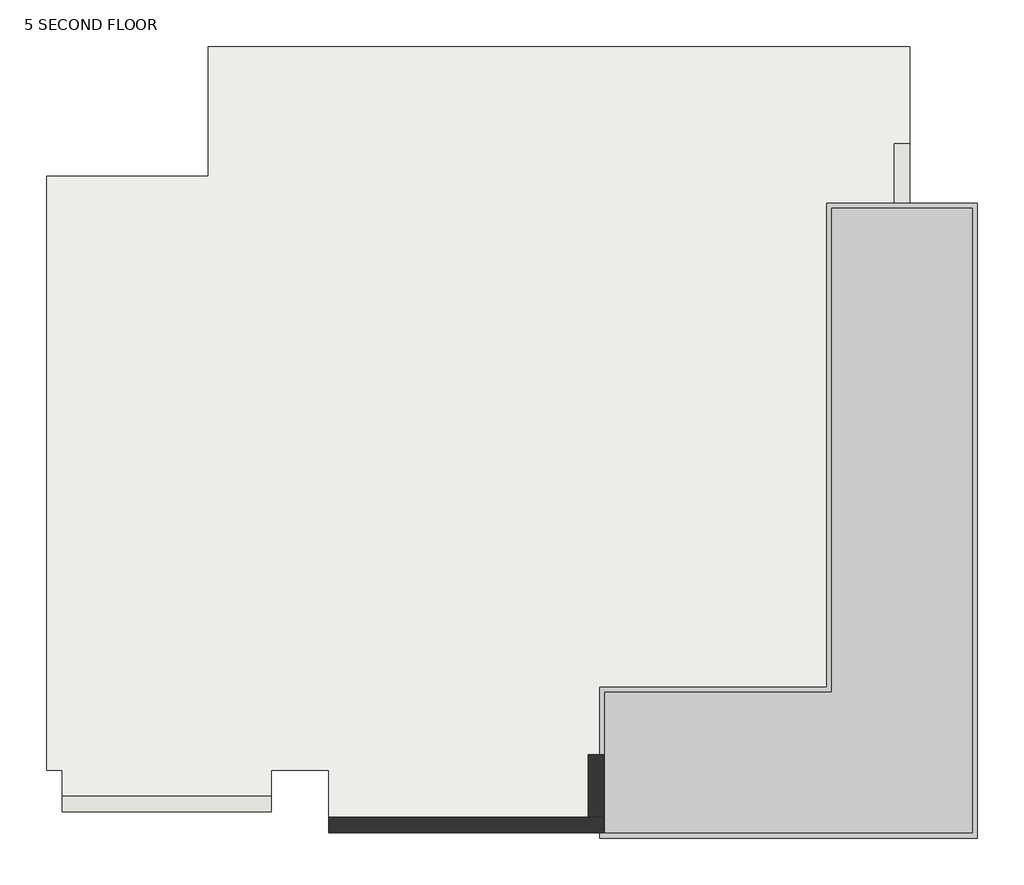
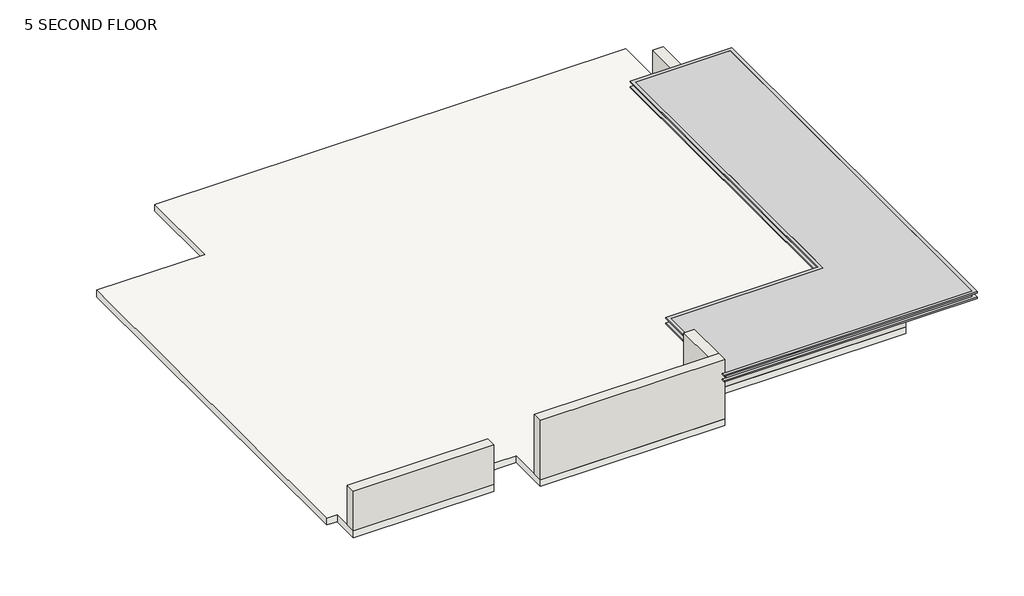
# One storey: 5 walls, 1 proxy, 1 slab.
"""IFC4 building model written with IfcOpenShell, lengths in millimetres."""

from ifc_helpers import new_model, si_unit, frame, origin, place, context, project, spatial, polyline, outline, extrude, faceted_brep, transform, mapped, element, save
from components import generic_models_3_generic_models_3_71c6270e

model = new_model("IFC4")

# Units and contexts
model_context = context("Model", 3, world=origin())
ifc_project = project(units=[si_unit("LENGTHUNIT", "METRE", prefix="MILLI")], contexts=[model_context])

# Site, building, storey
site = spatial("IfcSite", under=ifc_project)
building = spatial("IfcBuilding", under=site)
storey = spatial("IfcBuildingStorey", under=building, Name="5 SECOND FLOOR", Elevation=6858.0)

# Proxy
placement = place(None, origin())
generic_models_3_generic_models_3_shape = generic_models_3_generic_models_3_71c6270e(model_context)
element("IfcBuildingElementProxy", 1, Name="Generic Models 3 : Generic Models 3", ObjectType="Generic Models 3 : Generic Models 3", at=placement, inside=storey, context=model_context, shape_type="MappedRepresentation", body=[
    mapped(generic_models_3_generic_models_3_shape, transform((0.0, 0.0, 0.0), x_axis=(1.0, 0.0, 0.0), y_axis=(0.0, 1.0, 0.0), z_axis=(0.0, 0.0, 1.0))),
])

# Slab
element("IfcSlab", 2, ObjectType="ROOF", at=placement, inside=storey, context=model_context, shape_type="SweptSolid", body=[
    extrude(outline(polyline([(-5084.2350579, -7961.058484), (-5084.2350579, 733.2452215), (-2719.8942549, 733.2452215), (-2719.8942549, 2634.9534118), (7553.0590234, 2634.9534118), (7553.0590234, -7961.058484), (3071.3057451, -7961.058484), (3071.3057451, -8875.458484), (-954.5942549, -8875.458484), (-954.5942549, -7961.058484), (-1792.7942549, -7961.058484), (-1792.7942549, -8570.658484), (-4855.6350579, -8570.658484), (-4855.6350579, -7961.058484), (-5084.2350579, -7961.058484)])), frame((0.0, 0.0, 6705.6), z_axis=(0.0, 0.0, 1.0), x_axis=(1.0, 0.0, 0.0)), (0.0, 0.0, 1.0), 152.4),
])

# Walls
element("IfcWall", 3, ObjectType="9\"", at=placement, inside=storey, context=model_context, shape_type="SweptSolid", body=[
    extrude(outline(polyline([(-1792.7942549, -8570.658484), (-4855.6350579, -8570.658484), (-4855.6350579, -8342.058484), (-1792.7942549, -8342.058484), (-1792.7942549, -8570.658484)])), frame((0.0, 0.0, 6858.0), z_axis=(0.0, 0.0, 1.0), x_axis=(1.0, 0.0, 0.0)), (0.0, 0.0, 1.0), 914.4),
])
element("IfcWall", 4, ObjectType="9\"", at=placement, inside=storey, context=model_context, shape_type="Brep", body=[
    faceted_brep([(-954.5942549, -8875.458484, 6858.0), (3071.3057451, -8875.458484, 6858.0), (3071.3057451, -8875.458484, 8229.6), (-954.5942549, -8875.458484, 8229.6), (-954.5942549, -8646.858484, 6858.0), (-954.5942549, -8646.858484, 8229.6), (2842.7057451, -8646.858484, 8229.6), (3071.3057451, -8646.858484, 8229.6), (3071.3057451, -8646.858484, 6858.0), (2842.7057451, -8646.858484, 6858.0)], [[[0, 1, 2, 3]], [[4, 5, 6, 7, 8, 9]], [[1, 0, 4, 9, 8]], [[3, 2, 7, 6, 5]], [[0, 3, 5, 4]], [[2, 1, 8, 7]]]),
])
element("IfcWall", 5, ObjectType="9\"", at=placement, inside=storey, context=model_context, shape_type="Brep", body=[
    faceted_brep([(3071.3057451, -8646.858484, 6858.0), (3071.3057451, -7961.058484, 6858.0), (3071.3057451, -7732.458484, 6858.0), (3071.3057451, -7732.458484, 7772.4), (3071.3057451, -7732.458484, 8229.6), (3071.3057451, -8646.858484, 8229.6), (2842.7057451, -8646.858484, 6858.0), (2842.7057451, -8646.858484, 8229.6), (2842.7057451, -7732.458484, 8229.6), (2842.7057451, -7732.458484, 6858.0)], [[[0, 1, 2, 3, 4, 5]], [[6, 7, 8, 9]], [[2, 1, 0, 6, 9]], [[5, 4, 8, 7]], [[0, 5, 7, 6]], [[4, 3, 2, 9, 8]]]),
])
element("IfcWall", 6, ObjectType="9\"", at=placement, inside=storey, context=model_context, shape_type="Brep", body=[
    faceted_brep([(3071.3057451, -7961.058484, 6858.0), (7553.0590234, -7961.058484, 6858.0), (7553.0590234, -7961.058484, 7772.4), (3071.3057451, -7961.058484, 7772.4), (3071.3057451, -7732.458484, 6858.0), (3071.3057451, -7732.458484, 7772.4), (7324.4590234, -7732.458484, 7772.4), (7553.0590234, -7732.458484, 7772.4), (7553.0590234, -7732.458484, 6858.0), (7324.4590234, -7732.458484, 6858.0)], [[[0, 1, 2, 3]], [[4, 5, 6, 7, 8, 9]], [[1, 0, 4, 9, 8]], [[3, 2, 7, 6, 5]], [[0, 3, 5, 4]], [[2, 1, 8, 7]]]),
])
element("IfcWall", 7, ObjectType="9\"", at=placement, inside=storey, context=model_context, shape_type="SweptSolid", body=[
    extrude(outline(polyline([(7553.0590234, 1208.341516), (7553.0590234, -7732.458484), (7324.4590234, -7732.458484), (7324.4590234, 1208.341516), (7553.0590234, 1208.341516)])), frame((0.0, 0.0, 6858.0), z_axis=(0.0, 0.0, 1.0), x_axis=(1.0, 0.0, 0.0)), (0.0, 0.0, 1.0), 914.4),
])

save(model, "model.ifc")

# Revit data of these elements
# Type "ROOF"
#   Assembly Code = "B1010"
#   Function = 0
#   Layers, outside or top first: 0' - 6" no material (function 1)
# Type "9\""
#   Assembly Code = "B2010"
#   Layers, outside or top first: 0' - 9" no material (function 1)
# Element 1 (IfcBuildingElementProxy, "Generic Models 3 : Generic Models 3")
#   Phase Created = New Construction
#   Materials on its faces: "blk", "Topo cama"
# Element 2 (IfcSlab, "ROOF")
#   built-in parameter 1001955 = -1.5708 (stored number, unit not read)
#   Height Offset From Level = 0' - 0"
#   Phase Created = New Construction
#   Materials on its faces: "Default Floor", "st wall"
# Elements 3, 6, 7 (IfcWall, "9\"")
#   Top Offset = 0' - 0"
#   Base Offset = 0' - 0"
#   Unconnected Height = 3' - 0"
#   wall height = 3' - 0"
#   Phase Created = New Construction
#   Base Constraint = 5 SECOND FLOOR
#   Materials on its faces: "Default Wall"
# Element 4 (IfcWall, "9\"")
#   Top Offset = 0' - 0"
#   Base Offset = 0' - 0"
#   Unconnected Height = 4' - 6"
#   wall height = 4' - 6"
#   Phase Created = New Construction
#   Base Constraint = 5 SECOND FLOOR
#   Materials on its faces: "st wall", "Default Wall"
# Element 5 (IfcWall, "9\"")
#   Top Offset = 0' - 0"
#   Base Offset = 0' - 0"
#   Unconnected Height = 4' - 6"
#   wall height = 4' - 6"
#   Phase Created = New Construction
#   Base Constraint = 5 SECOND FLOOR
#   Materials on its faces: "Default Wall", "st wall"
# Materials
#   "blk": class "Generic", colour RGB 0 0 0, transparency 0, Cost = 0
#   "Topo cama": class "Wood", colour RGB 65 50 39, transparency 0
#   "Default Floor": colour RGB 128 128 128, transparency 0, Cost = 0
#   "st wall": class "Generic", colour RGB 85 49 28, transparency 0, Cost = 0
#   "Default Wall": colour RGB 128 128 128, transparency 0, Cost = 0
